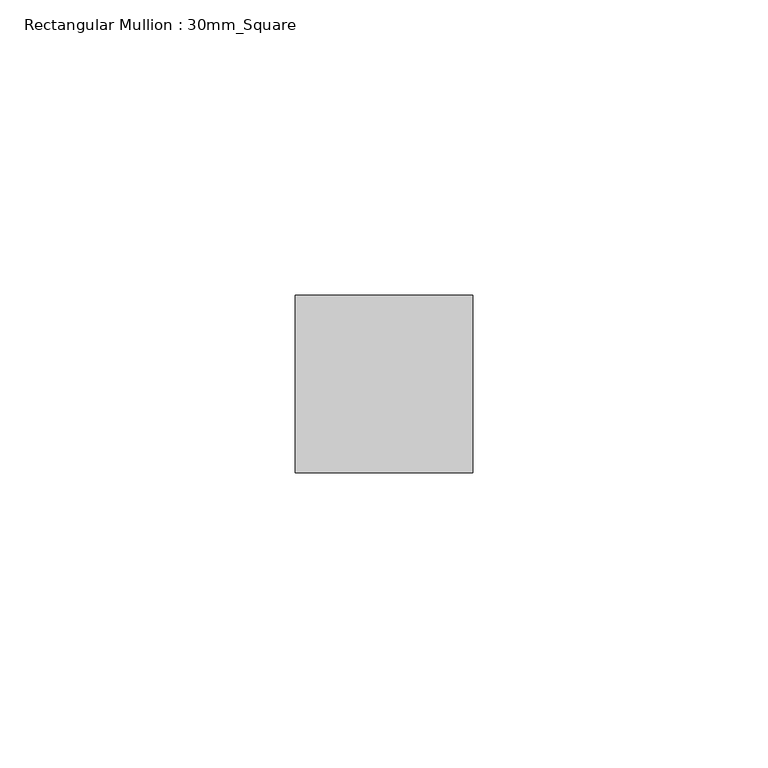
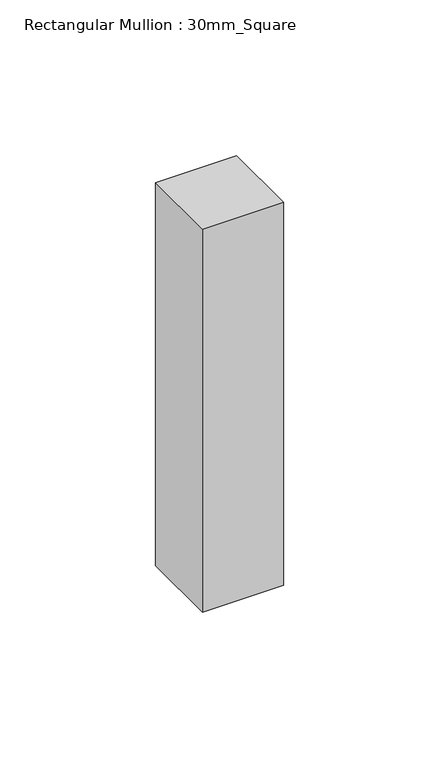
"""IFC4 building model written with IfcOpenShell, lengths in millimetres: member geometry, Rectangular Mullion : 30mm_Square."""

from ifc_helpers import new_model, si_unit, frame, origin, place, context, project, spatial, polyline, outline, extrude, source, transform, mapped, element, save


def rectangular_mullion_30mm_square_28ebc8b3(model_context):
    return source(origin(), model_context, "Body", "SweptSolid", [
        extrude(outline(polyline([(0.0, 15.0), (0.0, -15.0), (-30.0, -15.0), (-30.0, 15.0), (0.0, 15.0)])), frame((0.0, 0.0, -150.0429688), z_axis=(0.0, 0.0, 1.0), x_axis=(1.0, 0.0, 0.0)), (0.0, 0.0, 1.0), 150.0429688),
    ])


if __name__ == "__main__":
    model = new_model("IFC4")
    model_context = context("Model", 3, world=origin())
    ifc_project = project(units=[si_unit("LENGTHUNIT", "METRE", prefix="MILLI")], contexts=[model_context])
    site = spatial("IfcSite", under=ifc_project)
    building = spatial("IfcBuilding", under=site)
    placement = place(None, origin())
    rectangular_mullion_30mm_square_shape = rectangular_mullion_30mm_square_28ebc8b3(model_context)
    element("IfcMember", 1, ObjectType="Rectangular Mullion : 30mm_Square", at=placement, inside=building, context=model_context, shape_type="MappedRepresentation", body=[
        mapped(rectangular_mullion_30mm_square_shape, transform((0.0, 0.0, 0.0), x_axis=(1.0, 0.0, 0.0), y_axis=(0.0, 1.0, 0.0), z_axis=(0.0, 0.0, 1.0))),
    ])
    save(model, "model.ifc")

# Revit data of these elements
# Type "Rectangular Mullion : 30mm_Square"
#   Keynote = "H11"
#   built-in parameter 1007304 = 0.0984252 (stored number, unit not read)
#   built-in parameter 1007301 = 0.0492126 (stored number, unit not read)
#   built-in parameter 1007300 = 0.0492126 (stored number, unit not read)
# Element 1 (IfcMember, "Rectangular Mullion : 30mm_Square")
#   Materials on its faces: "Aluminium"
# Materials
#   "Aluminium": class "Metal", colour RGB 247 247 247, transparency 0, Description = "Aluminium 6061", Cost = 0
